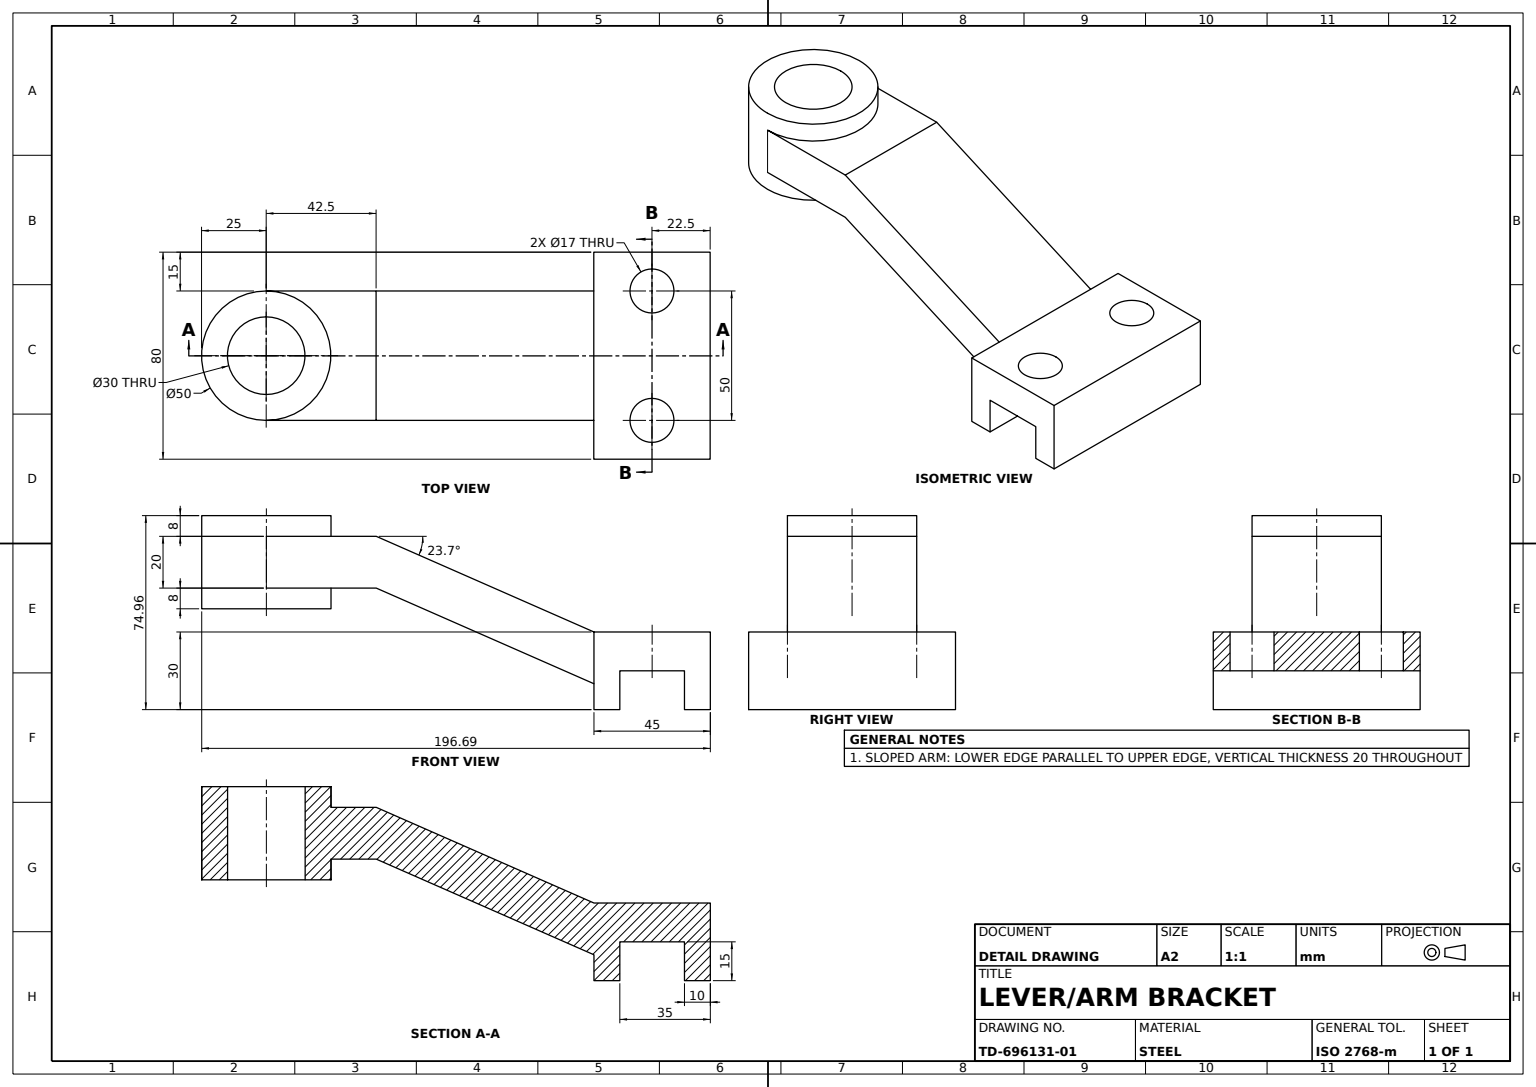
from build123d import *

# Parameters (mm, degrees)
ARM_BODY_DEPTH            = 80
END_BLOCK_DEPTH           = 60
END_BLOCK_SLOT_CUT_DEPTH  = 15
END_BLOCK_PAD_5MM_DEPTH   = 5
MOUNTING_HOLES_SKETCH_R   = 8.5
MOUNTING_HOLES_2X_DEPTH   = 15
ARM_RELIEF_CUT_DEPTH      = 55
ARM_WEB_SKETCH_W          = 42.5
ARM_WEB_SKETCH_H          = 20
ARM_WEB_DEPTH             = 50
HUB_FLANGE_LOWER_SKETCH_R = 25
HUB_FLANGE_LOWER_50_DEPTH = 8
HUB_START                 = 20
HUB_BODY_DEPTH            = 20
HUB_START_2               = 8
HUB_FLANGE_UPPER_SKETCH_R = 25
HUB_FLANGE_UPPER_50_DEPTH = 8
HUB_BORE_SKETCH_R         = 15
HUB_BORE_30_DEPTH         = 40


with BuildPart() as part:
    # Arm Profile Sketch → Arm Body (new body)
    with BuildSketch(Plane.XY):
        Polygon((0, 0), (10, 0), (10, 15), (35, 15), (35, 0), (45, 0), (45, 30), (0, 30), align=None)
    extrude(amount=ARM_BODY_DEPTH)

    # End Block Sketch → End Block (add)
    with BuildSketch(Plane.XY.offset(80)):
        Polygon((-102.5, 75), (-102.5, 55), (0, 10), (0, 30), align=None)
    extrude(amount=-END_BLOCK_DEPTH)

    # End Block Slot Sketch → End Block Slot Cut (cut)
    with BuildSketch(Plane.XY.offset(80)):
        Polygon((-102.5, 75), (0, 30), (0, 10), (-102.5, 55), align=None)
    extrude(amount=-END_BLOCK_SLOT_CUT_DEPTH, mode=Mode.SUBTRACT)

    # End Block Pad Sketch → End Block Pad 5mm (add)
    with BuildSketch(Plane(origin=(0, 0, 20), x_dir=(-1, 0, 0), z_dir=(0, 0, -1))):
        Polygon((0, 30), (102.5, 75), (102.5, 55), (0, 10), align=None)
    extrude(amount=END_BLOCK_PAD_5MM_DEPTH)

    # Mounting Holes Sketch → Mounting Holes 2x (cut)
    with BuildSketch(Plane(origin=(0, 30, 0), x_dir=(1, 0, 0), z_dir=(0, 1, 0))):
        with Locations(Location((22.5, -15, 0), (0, 0, 270))):
            Circle(MOUNTING_HOLES_SKETCH_R)
        with Locations(Location((22.5, -65, 0), (0, 0, 270))):
            Circle(MOUNTING_HOLES_SKETCH_R)
    extrude(amount=-MOUNTING_HOLES_2X_DEPTH, mode=Mode.SUBTRACT)

    # Arm Relief Cut Sketch → Arm Relief Cut (cut)
    with BuildSketch(Plane.XY.offset(65)):
        Polygon((-102.5, 75), (-84.187119396, 66.960198759), (-84.187119396, 46.960198759), (-102.5, 55), align=None)
    extrude(amount=-ARM_RELIEF_CUT_DEPTH, mode=Mode.SUBTRACT)

    # Arm Web Sketch → Arm Web (add)
    with BuildSketch(Plane.XY.offset(65)):
        with Locations((-105.437119396, 56.960198759)):
            Rectangle(ARM_WEB_SKETCH_W, ARM_WEB_SKETCH_H)
    extrude(amount=-ARM_WEB_DEPTH)

    # Hub Flange Lower Sketch → Hub Flange Lower Ø50 (add)
    with BuildSketch(Plane(origin=(0, 66.960198759, 0), x_dir=(1, 0, 0), z_dir=(0, 1, 0))):
        with Locations(Location((-126.687119396, -40, 0), (0, 0, 270))):
            Circle(HUB_FLANGE_LOWER_SKETCH_R)
    extrude(amount=HUB_FLANGE_LOWER_50_DEPTH)

    # Hub Body Sketch → Hub Body (add)
    with BuildSketch(Plane.XZ.offset(-66.960198759).offset(HUB_START)):
        with BuildLine():
            Line((-126.687119396, 65), (-126.687119396, 15))
            ThreePointArc((-126.687119396, 15), (-151.687119396, 40), (-126.687119396, 65))
        make_face()
    extrude(amount=-HUB_BODY_DEPTH)

    # Hub Flange Upper Sketch → Hub Flange Upper Ø50 (add)
    with BuildSketch(Plane.XZ.offset(-46.960198759).offset(HUB_START_2)):
        with Locations(Location((-126.687119396, 40, 0), (0, 0, 270))):
            Circle(HUB_FLANGE_UPPER_SKETCH_R)
    extrude(amount=-HUB_FLANGE_UPPER_50_DEPTH)

    # Hub Bore Sketch → Hub Bore Ø30 (cut)
    with BuildSketch(Plane(origin=(0, 74.960198759, 0), x_dir=(1, 0, 0), z_dir=(0, 1, 0))):
        with Locations(Location((-126.687119396, -40, 0), (0, 0, 270))):
            Circle(HUB_BORE_SKETCH_R)
    extrude(amount=-HUB_BORE_30_DEPTH, mode=Mode.SUBTRACT)


solid = part.part
